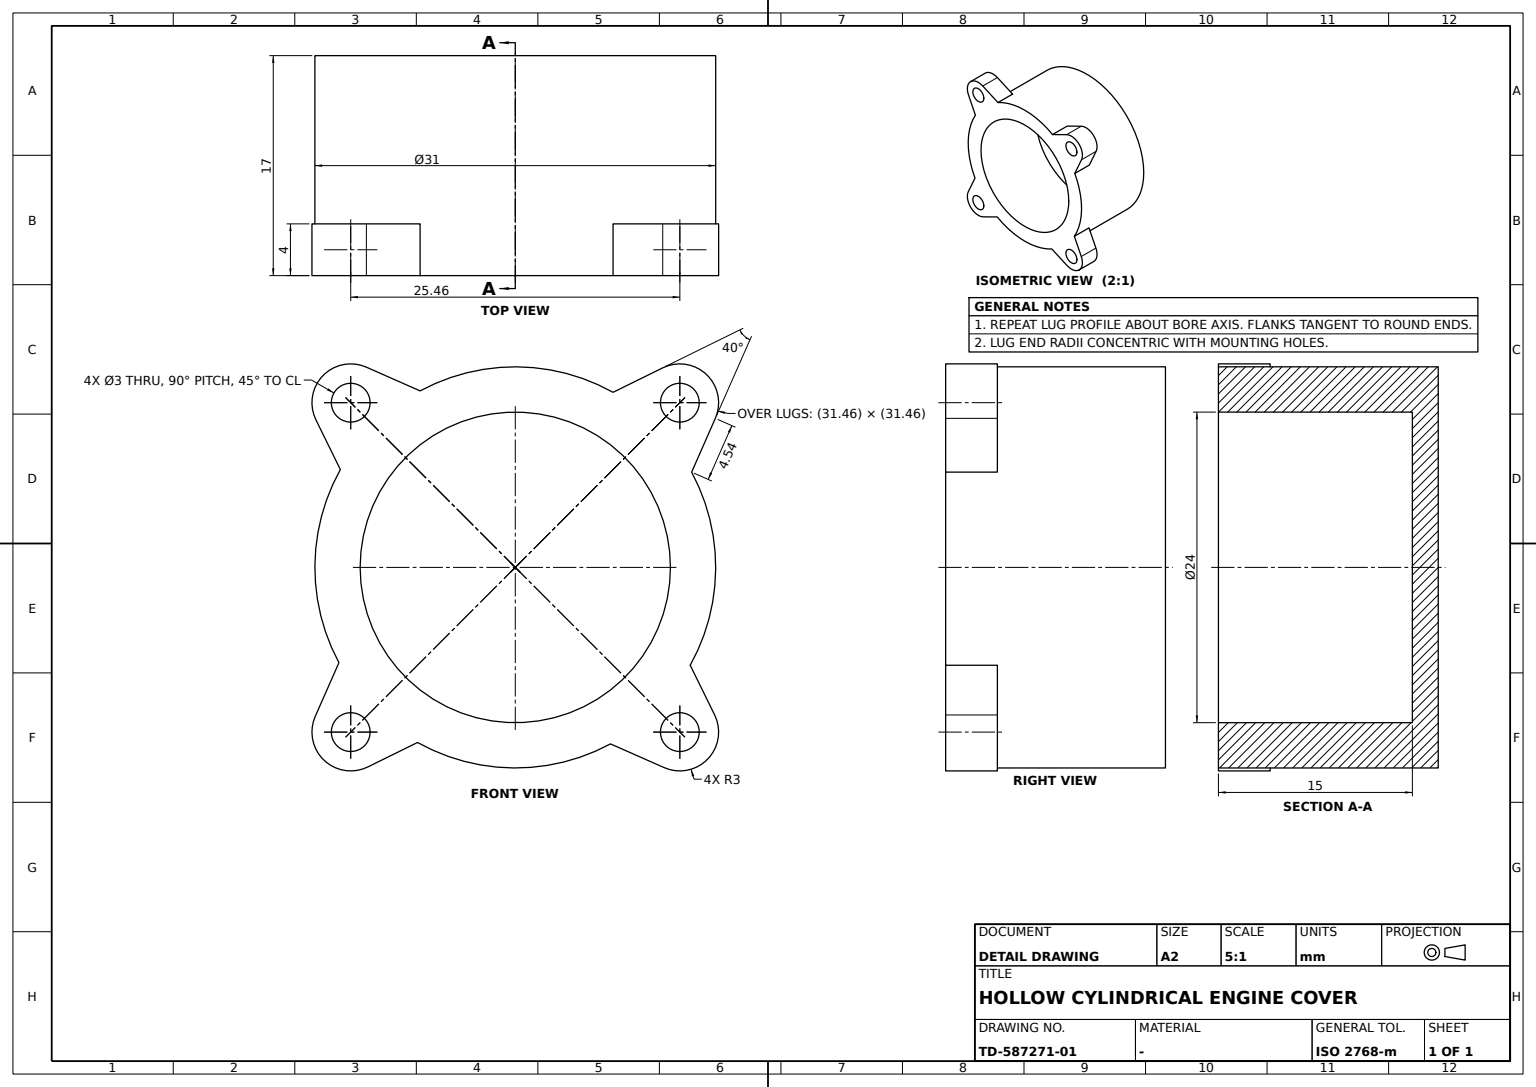
CATIA V5 part; units mm, degrees
sketch "Sketch1" plane through (0, 0, 0) normal (0, 0, 1) x (0, 1, 0)
  circle A0 centre (0, 0) radius 15.5
  dimension "radius A0" = 15.5
extrude "Pad1" add sketch "Sketch1" along normal blind 17
sketch "Sketch2" plane through (0, 0, 17) normal (0, 0, 1) x (1, 0, 0)
  circle A0 centre (0, 0) radius 12
  dimension "radius A0" = 12
extrude "Pocket1" cut sketch "Sketch2" against normal blind 15
sketch "Sketch3" plane through (0, 0, 17) normal (0, 0, 1) x (0, 1, 0)
  point P0 (3.4327, 11.4985)
  line L0 (3.4327, 11.4985) -> (11.4037, 15.4198)
  arc A0 (11.4037, 15.4198) -> (15.4727, 11.517) centre (12.7279, 12.7279) cw
  point P1 (12.7279, 12.7279)
  line L1 (15.4727, 11.517) -> (11.654, 2.861)
  point P2 (11.654, 2.861)
  circle A1 centre (0, 0) radius 12 construction
  circle A2 centre (0, 0) radius 12 construction
  circle A3 centre (12.7279, 12.7279) radius 1.5
  line L2 (0, 0) -> (18.1446, 18.1446) construction
  arc A4 (11.654, 2.861) -> (3.4327, 11.4985) centre (0, 0) ccw
  dimension "radius A0" = 3
  dimension "radius A3" = 1.5
  dimension "angle L2 x axis" = 45
  dimension "angle L1 L0" = 40
  dimension "distance origin P1" = 18
  dimension "length L1" = 9.4609
  constraint tangency A0 L0
  constraint tangency L1 A0
  constraint coincidence P0 A1
  constraint coincidence P2 A2
  constraint coincidence P1 L2
  constraint concentricity A3 A0
extrude "Pad2" add sketch "Sketch3" against normal blind 4
pattern_circular "CircPattern1" count 4 over 360 about axis through (0, 0, 17) along (0, 0, 1) of "Pad2"
equation "\"angular step@CircPattern1\" = 360.0*1 deg/CircPattern1.AngularNumber"
